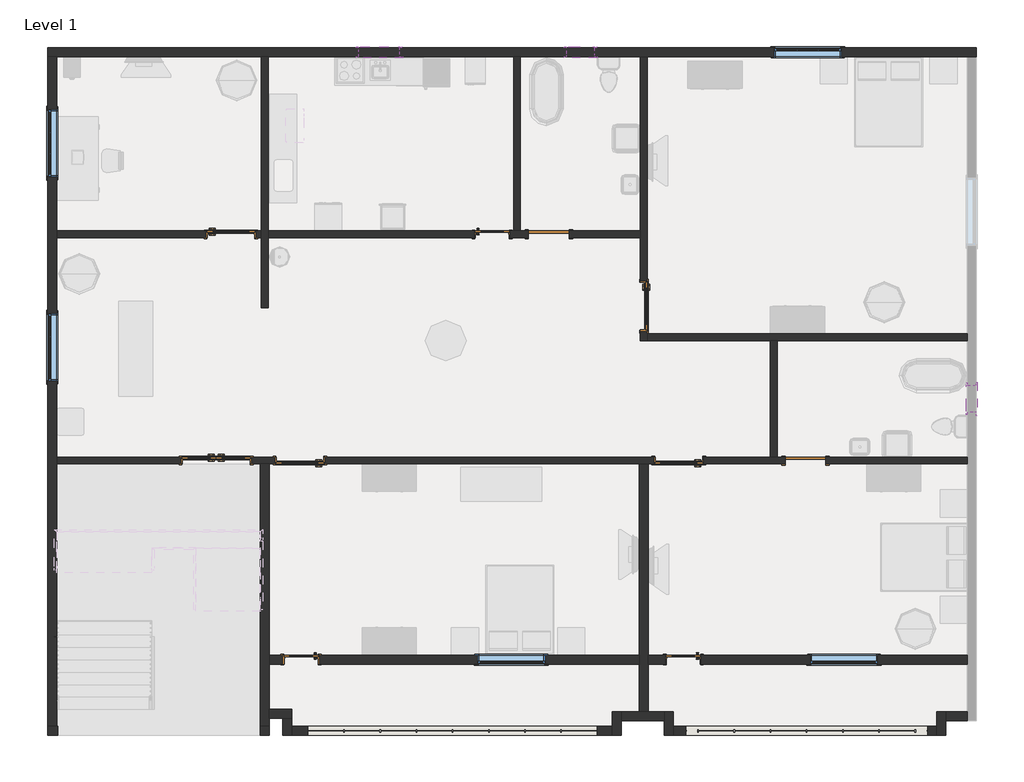
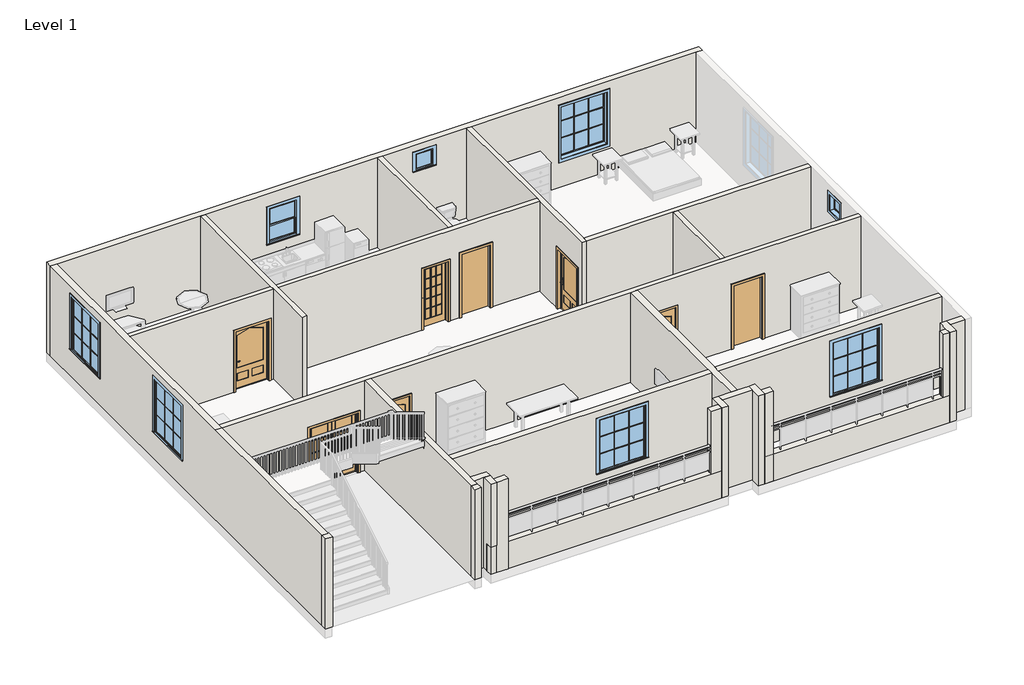
# One storey, part 1 of 4: 27 walls, 10 doors, 8 windows.
"""IFC4 building model written with IfcOpenShell, lengths in millimetres."""

from ifc_helpers import new_model, si_unit, frame, origin, origin_with_axes, place, context, project, spatial, polyline, outline, extrude, faceted_brep, transform, mapped, element, save
from components import door_25c67de5, door_94998e6c, door_d788789e, door_fa41f557, door_686f89d2, window_cc15f82e, window_1554aedb, window_e41d21a6

model = new_model("IFC4")

# Units and contexts
model_context = context("Model", 3, world=origin())
ifc_project = project(units=[si_unit("LENGTHUNIT", "METRE", prefix="MILLI")], contexts=[model_context])

# Site, building, storey
site = spatial("IfcSite", under=ifc_project)
building = spatial("IfcBuilding", under=site)
storey = spatial("IfcBuildingStorey", under=building, Name="Level 1", Elevation=0.0)

# Doors
placement = place(None, origin())
door_shape = door_25c67de5(model_context)
element("IfcDoor", 1, ObjectType="42\" x 80\"", at=placement, inside=storey, context=model_context, shape_type="MappedRepresentation", body=[
    mapped(door_shape, transform((-14516.2480019, 5391.0508877, 0.0), x_axis=(1.0, 0.0, 0.0), y_axis=(0.0, 1.0, 0.0), z_axis=(0.0, 0.0, 1.0))),
])
element("IfcDoor", 2, ObjectType="42\" x 80\"", at=placement, inside=storey, context=model_context, shape_type="MappedRepresentation", body=[
    mapped(door_shape, transform((-6007.2480019, 5391.0508877, 0.0), x_axis=(1.0, 0.0, 0.0), y_axis=(0.0, 1.0, 0.0), z_axis=(0.0, 0.0, 1.0))),
])
element("IfcDoor", 3, ObjectType="42\" x 80\"", at=placement, inside=storey, context=model_context, shape_type="MappedRepresentation", body=[
    mapped(door_shape, transform((-16065.6480019, 10477.4008877, 0.0), x_axis=(-1.0, 0.0, 0.0), y_axis=(0.0, -1.0, 0.0), z_axis=(0.0, 0.0, 1.0))),
])
element("IfcDoor", 4, ObjectType="42\" x 80\"", at=placement, inside=storey, context=model_context, shape_type="MappedRepresentation", body=[
    mapped(door_shape, transform((-6791.4730019, 8861.3258877, 0.0), x_axis=(0.0, 1.0, 0.0), y_axis=(-1.0, 0.0, 0.0), z_axis=(0.0, 0.0, 1.0))),
])
door_2_shape = door_94998e6c(model_context)
element("IfcDoor", 5, ObjectType="Door-Exterior-Double-Full Glass-Wood_Clad : 60\" x 80\"", at=placement, inside=storey, context=model_context, shape_type="MappedRepresentation", body=[
    mapped(door_2_shape, transform((-16395.8480019, 5397.4008877, 0.0), x_axis=(1.0, 0.0, 0.0), y_axis=(0.0, 1.0, 0.0), z_axis=(0.0, 0.0, 1.0))),
])
door_3_shape = door_d788789e(model_context)
element("IfcDoor", 6, ObjectType="Door-Interior-Single-Full Glass-Wood : 30\" x 80\"", at=placement, inside=storey, context=model_context, shape_type="MappedRepresentation", body=[
    mapped(door_3_shape, transform((-14490.8480019, 927.0008877, 0.0), x_axis=(-1.0, 0.0, 0.0), y_axis=(0.0, -1.0, 0.0), z_axis=(0.0, 0.0, 1.0))),
])
element("IfcDoor", 7, ObjectType="Door-Interior-Single-Full Glass-Wood : 30\" x 80\"", at=placement, inside=storey, context=model_context, shape_type="MappedRepresentation", body=[
    mapped(door_3_shape, transform((-5905.6480019, 927.0008877, 0.0), x_axis=(-1.0, 0.0, 0.0), y_axis=(0.0, -1.0, 0.0), z_axis=(0.0, 0.0, 1.0))),
])
door_4_shape = door_fa41f557(model_context)
element("IfcDoor", 8, ObjectType="Door-Interior-Single-Full Glass-Wood : 30\" x 80\"", at=placement, inside=storey, context=model_context, shape_type="MappedRepresentation", body=[
    mapped(door_4_shape, transform((-10198.2480019, 10477.4008877, 0.0), x_axis=(1.0, 0.0, 0.0), y_axis=(0.0, 1.0, 0.0), z_axis=(0.0, 0.0, 1.0))),
])
door_5_shape = door_686f89d2(model_context)
element("IfcDoor", 9, ObjectType="Single-Flush : 36\" x 84\"", at=placement, inside=storey, context=model_context, shape_type="MappedRepresentation", body=[
    mapped(door_5_shape, transform((-8928.2480019, 10474.2258877, 0.0), x_axis=(-1.0, 0.0, 0.0), y_axis=(0.0, -1.0, 0.0), z_axis=(0.0, 0.0, 1.0))),
])
element("IfcDoor", 10, ObjectType="Single-Flush : 36\" x 84\"", at=placement, inside=storey, context=model_context, shape_type="MappedRepresentation", body=[
    mapped(door_5_shape, transform((-3162.4480019, 5394.2258877, 0.0), x_axis=(-1.0, 0.0, 0.0), y_axis=(0.0, -1.0, 0.0), z_axis=(0.0, 0.0, 1.0))),
])

# Walls
element("IfcWall", 11, ObjectType="Generic - 8\"", at=placement, inside=storey, context=model_context, shape_type="Brep", body=[
    faceted_brep([(-20180.4480019, 14462.0258877, 0.0), (-19977.2480019, 14462.0258877, 0.0), (-15379.8480019, 14462.0258877, 0.0), (-15227.4480019, 14462.0258877, 0.0), (-9715.6480019, 14462.0258877, 0.0), (-9563.2480019, 14462.0258877, 0.0), (-6870.8480019, 14462.0258877, 0.0), (-6718.4480019, 14462.0258877, 0.0), (469.7519981, 14462.0258877, 0.0), (672.9519981, 14462.0258877, 0.0), (672.9519981, 14462.0258877, 3048.0), (469.7519981, 14462.0258877, 3048.0), (-6718.4480019, 14462.0258877, 3048.0), (-6870.8480019, 14462.0258877, 3048.0), (-9563.2480019, 14462.0258877, 3048.0), (-9715.6480019, 14462.0258877, 3048.0), (-15227.4480019, 14462.0258877, 3048.0), (-15379.8480019, 14462.0258877, 3048.0), (-19977.2480019, 14462.0258877, 3048.0), (-20180.4480019, 14462.0258877, 3048.0), (-2349.6480019, 14462.0258877, 2743.2), (-2349.6480019, 14462.0258877, 914.4), (-3873.6480019, 14462.0258877, 914.4), (-3873.6480019, 14462.0258877, 2743.2), (-8521.8480019, 14462.0258877, 2768.6), (-7912.2480019, 14462.0258877, 2768.6), (-7912.2480019, 14462.0258877, 2159.0), (-8521.8480019, 14462.0258877, 2159.0), (-13195.4480019, 14462.0258877, 2554.7223406), (-12281.0480019, 14462.0258877, 2554.7223406), (-12281.0480019, 14462.0258877, 1335.5223406), (-13195.4480019, 14462.0258877, 1335.5223406), (-20180.4480019, 14665.2258877, 0.0), (-20180.4480019, 14665.2258877, 3048.0), (672.9519981, 14665.2258877, 3048.0), (672.9519981, 14665.2258877, 0.0), (-2349.6480019, 14665.2258877, 2743.2), (-3873.6480019, 14665.2258877, 2743.2), (-3873.6480019, 14665.2258877, 914.4), (-2349.6480019, 14665.2258877, 914.4), (-8521.8480019, 14665.2258877, 2768.6), (-8521.8480019, 14665.2258877, 2159.0), (-7912.2480019, 14665.2258877, 2159.0), (-7912.2480019, 14665.2258877, 2768.6), (-13195.4480019, 14665.2258877, 2554.7223406), (-13195.4480019, 14665.2258877, 1335.5223406), (-12281.0480019, 14665.2258877, 1335.5223406), (-12281.0480019, 14665.2258877, 2554.7223406)], [[[0, 1, 2, 3, 4, 5, 6, 7, 8, 9, 10, 11, 12, 13, 14, 15, 16, 17, 18, 19], [20, 21, 22, 23], [24, 25, 26, 27], [28, 29, 30, 31]], [[32, 33, 34, 35], [36, 37, 38, 39], [40, 41, 42, 43], [44, 45, 46, 47]], [[9, 8, 7, 6, 5, 4, 3, 2, 1, 0, 32, 35]], [[0, 19, 33, 32]], [[10, 9, 35, 34]], [[21, 20, 36, 39]], [[22, 21, 39, 38]], [[23, 22, 38, 37]], [[20, 23, 37, 36]], [[41, 40, 24, 27]], [[42, 41, 27, 26]], [[43, 42, 26, 25]], [[40, 43, 25, 24]], [[45, 44, 28, 31]], [[46, 45, 31, 30]], [[47, 46, 30, 29]], [[44, 47, 29, 28]], [[19, 18, 17, 16, 15, 14, 13, 12, 11, 10, 34, 33]]]),
])
element("IfcWall", 12, ObjectType="Generic - 8\"", at=placement, inside=storey, context=model_context, shape_type="Brep", body=[
    faceted_brep([(-19977.2480019, -574.7741123, 0.0), (-19977.2480019, 5318.0258877, 0.0), (-19977.2480019, 5470.4258877, 0.0), (-19977.2480019, 10398.0258877, 0.0), (-19977.2480019, 10550.4258877, 0.0), (-19977.2480019, 14462.0258877, 0.0), (-19977.2480019, 14462.0258877, 3048.0), (-19977.2480019, 10550.4258877, 3048.0), (-19977.2480019, 10398.0258877, 3048.0), (-19977.2480019, 5470.4258877, 3048.0), (-19977.2480019, 5318.0258877, 3048.0), (-19977.2480019, -574.7741123, 3048.0), (-19977.2480019, 13280.9258877, 2743.2), (-19977.2480019, 13280.9258877, 914.4), (-19977.2480019, 11756.9258877, 914.4), (-19977.2480019, 11756.9258877, 2743.2), (-19977.2480019, 8696.2258877, 2743.2), (-19977.2480019, 8696.2258877, 914.4), (-19977.2480019, 7172.2258877, 914.4), (-19977.2480019, 7172.2258877, 2743.2), (-20180.4480019, -574.7741123, 0.0), (-20180.4480019, -574.7741123, 3048.0), (-20180.4480019, 5318.0258877, 3048.0), (-20180.4480019, 14462.0258877, 3048.0), (-20180.4480019, 14462.0258877, 0.0), (-20180.4480019, 13280.9258877, 2743.2), (-20180.4480019, 11756.9258877, 2743.2), (-20180.4480019, 11756.9258877, 914.4), (-20180.4480019, 13280.9258877, 914.4), (-20180.4480019, 8696.2258877, 2743.2), (-20180.4480019, 7172.2258877, 2743.2), (-20180.4480019, 7172.2258877, 914.4), (-20180.4480019, 8696.2258877, 914.4)], [[[0, 1, 2, 3, 4, 5, 6, 7, 8, 9, 10, 11], [12, 13, 14, 15], [16, 17, 18, 19]], [[20, 21, 22, 23, 24], [25, 26, 27, 28], [29, 30, 31, 32]], [[5, 4, 3, 2, 1, 0, 20, 24]], [[6, 5, 24, 23]], [[0, 11, 21, 20]], [[13, 12, 25, 28]], [[14, 13, 28, 27]], [[15, 14, 27, 26]], [[12, 15, 26, 25]], [[17, 16, 29, 32]], [[18, 17, 32, 31]], [[19, 18, 31, 30]], [[16, 19, 30, 29]], [[11, 10, 22, 21]], [[10, 9, 8, 7, 6, 23, 22]]]),
])
element("IfcWall", 13, ObjectType="Generic - 8\"", at=placement, inside=storey, context=model_context, shape_type="Brep", body=[
    faceted_brep([(-15202.0480019, -574.7741123, 0.0), (-15202.0480019, -396.9741123, 0.0), (-15202.0480019, -193.7741123, 0.0), (-15202.0480019, 822.2258877, 0.0), (-15202.0480019, 1025.4258877, 0.0), (-15202.0480019, 5318.0258877, 0.0), (-15202.0480019, 5318.0258877, 3048.0), (-15202.0480019, 1025.4258877, 3048.0), (-15202.0480019, 822.2258877, 3048.0), (-15202.0480019, -193.7741123, 3048.0), (-15202.0480019, -396.9741123, 3048.0), (-15202.0480019, -574.7741123, 3048.0), (-15405.2480019, -574.7741123, 0.0), (-15405.2480019, -574.7741123, 3048.0), (-15405.2480019, 5318.0258877, 3048.0), (-15405.2480019, 5318.0258877, 0.0)], [[[0, 1, 2, 3, 4, 5, 6, 7, 8, 9, 10, 11]], [[12, 13, 14, 15]], [[5, 4, 3, 2, 1, 0, 12, 15]], [[0, 11, 13, 12]], [[6, 5, 15, 14]], [[11, 10, 9, 8, 7, 6, 14, 13]]]),
])
element("IfcWall", 14, ObjectType="Generic - 8\"", at=placement, inside=storey, context=model_context, shape_type="SweptSolid", body=[
    extrude(outline(polyline([(3048.0, -15202.0480019), (0.0, -15202.0480019), (0.0, -14897.2480019), (2057.4, -14897.2480019), (2057.4, -14084.4480019), (0.0, -14084.4480019), (0.0, -6896.2480019), (3048.0, -6896.2480019), (3048.0, -15202.0480019)]), holes=[polyline([(914.4, -10528.4480019), (2743.2, -10528.4480019), (2743.2, -9004.4480019), (914.4, -9004.4480019), (914.4, -10528.4480019)])]), frame((0.0, 822.2258877, 0.0), z_axis=(0.0, 1.0, 0.0), x_axis=(0.0, 0.0, 1.0)), (0.0, 0.0, 1.0), 203.2),
    extrude(outline(polyline([(0.0, 469.7519981), (3048.0, 469.7519981), (3048.0, -6693.0480019), (0.0, -6693.0480019), (0.0, -6312.0480019), (2057.4, -6312.0480019), (2057.4, -5499.2480019), (0.0, -5499.2480019), (0.0, 469.7519981)]), holes=[polyline([(914.4, -3060.8480019), (2743.2, -3060.8480019), (2743.2, -1536.8480019), (914.4, -1536.8480019), (914.4, -3060.8480019)])]), frame((0.0, 822.2258877, 0.0), z_axis=(0.0, 1.0, 0.0), x_axis=(0.0, 0.0, 1.0)), (0.0, 0.0, 1.0), 203.2),
])
element("IfcWall", 15, ObjectType="Generic - 8\"", at=placement, inside=storey, context=model_context, shape_type="Brep", body=[
    faceted_brep([(-15202.0480019, -396.9741123, 0.0), (-14897.2480019, -396.9741123, 0.0), (-14694.0480019, -396.9741123, 0.0), (-14694.0480019, -396.9741123, 3048.0), (-14897.2480019, -396.9741123, 3048.0), (-15202.0480019, -396.9741123, 3048.0), (-15202.0480019, -193.7741123, 0.0), (-15202.0480019, -193.7741123, 3048.0), (-14694.0480019, -193.7741123, 3048.0), (-14694.0480019, -193.7741123, 0.0)], [[[0, 1, 2, 3, 4, 5]], [[6, 7, 8, 9]], [[2, 1, 0, 6, 9]], [[0, 5, 7, 6]], [[3, 2, 9, 8]], [[5, 4, 3, 8, 7]]]),
])
element("IfcWall", 16, ObjectType="Generic - 8\"", at=placement, inside=storey, context=model_context, shape_type="Brep", body=[
    faceted_brep([(-14897.2480019, -396.9741123, 0.0), (-14897.2480019, -574.7741123, 0.0), (-14897.2480019, -574.7741123, 914.4), (-14897.2480019, -777.9741123, 914.4), (-14897.2480019, -777.9741123, 3048.0), (-14897.2480019, -396.9741123, 3048.0), (-14694.0480019, -396.9741123, 0.0), (-14694.0480019, -396.9741123, 3048.0), (-14694.0480019, -574.7741123, 3048.0), (-14694.0480019, -777.9741123, 3048.0), (-14694.0480019, -777.9741123, 914.4), (-14694.0480019, -574.7741123, 914.4), (-14694.0480019, -574.7741123, 0.0)], [[[0, 1, 2, 3, 4, 5]], [[6, 7, 8, 9, 10, 11, 12]], [[1, 0, 6, 12]], [[0, 5, 7, 6]], [[10, 3, 2, 11]], [[2, 1, 12, 11]], [[4, 3, 10, 9]], [[5, 4, 9, 8, 7]]]),
])
element("IfcWall", 17, ObjectType="Generic - 8\"", at=placement, inside=storey, context=model_context, shape_type="SweptSolid", body=[
    extrude(outline(polyline([(-15405.2480019, -574.7741123), (-15202.0480019, -574.7741123), (-15202.0480019, -777.9741123), (-15405.2480019, -777.9741123), (-15405.2480019, -574.7741123)])), origin_with_axes(), (0.0, 0.0, 1.0), 3048.0),
])
element("IfcWall", 18, ObjectType="Generic - 8\"", at=placement, inside=storey, context=model_context, shape_type="Brep", body=[
    faceted_brep([(-7302.6480019, -777.9741123, 3048.0), (-7302.6480019, -777.9741123, 0.0), (-7302.6480019, -447.7741123, 0.0), (-7302.6480019, -244.5741123, 0.0), (-7302.6480019, -244.5741123, 3048.0), (-7302.6480019, -447.7741123, 3048.0), (-7505.8480019, -777.9741123, 0.0), (-7505.8480019, -777.9741123, 914.4), (-7505.8480019, -777.9741123, 3048.0), (-7505.8480019, -574.7741123, 3048.0), (-7505.8480019, -244.5741123, 3048.0), (-7505.8480019, -244.5741123, 0.0), (-7505.8480019, -574.7741123, 0.0)], [[[0, 1, 2, 3, 4, 5]], [[6, 7, 8, 9, 10, 11, 12]], [[3, 2, 1, 6, 12, 11]], [[4, 3, 11, 10]], [[0, 8, 7, 6, 1]], [[0, 5, 4, 10, 9, 8]]]),
])
element("IfcWall", 19, ObjectType="Generic - 8\"", at=placement, inside=storey, context=model_context, shape_type="Brep", body=[
    faceted_brep([(-7302.6480019, -447.7741123, 0.0), (-6337.4480019, -447.7741123, 0.0), (-6337.4480019, -447.7741123, 3048.0), (-7302.6480019, -447.7741123, 3048.0), (-7302.6480019, -244.5741123, 0.0), (-7302.6480019, -244.5741123, 3048.0), (-6896.2480019, -244.5741123, 3048.0), (-6693.0480019, -244.5741123, 3048.0), (-6337.4480019, -244.5741123, 3048.0), (-6337.4480019, -244.5741123, 0.0), (-6693.0480019, -244.5741123, 0.0), (-6896.2480019, -244.5741123, 0.0)], [[[0, 1, 2, 3]], [[4, 5, 6, 7, 8, 9, 10, 11]], [[1, 0, 4, 11, 10, 9]], [[0, 3, 5, 4]], [[2, 1, 9, 8]], [[3, 2, 8, 7, 6, 5]]]),
])
element("IfcWall", 20, ObjectType="Generic - 8\"", at=placement, inside=storey, context=model_context, shape_type="Brep", body=[
    faceted_brep([(-6337.4480019, -244.5741123, 0.0), (-6337.4480019, -447.7741123, 0.0), (-6337.4480019, -777.9741123, 0.0), (-6337.4480019, -777.9741123, 3048.0), (-6337.4480019, -447.7741123, 3048.0), (-6337.4480019, -244.5741123, 3048.0), (-6134.2480019, -244.5741123, 0.0), (-6134.2480019, -244.5741123, 3048.0), (-6134.2480019, -574.7741123, 3048.0), (-6134.2480019, -777.9741123, 3048.0), (-6134.2480019, -777.9741123, 914.4), (-6134.2480019, -777.9741123, 0.0), (-6134.2480019, -574.7741123, 0.0)], [[[0, 1, 2, 3, 4, 5]], [[6, 7, 8, 9, 10, 11, 12]], [[2, 1, 0, 6, 12, 11]], [[0, 5, 7, 6]], [[2, 11, 10, 9, 3]], [[5, 4, 3, 9, 8, 7]]]),
])
element("IfcWall", 21, ObjectType="Generic - 8\"", at=placement, inside=storey, context=model_context, shape_type="Brep", body=[
    faceted_brep([(-7505.8480019, -574.7741123, 0.0), (-14694.0480019, -574.7741123, 0.0), (-14897.2480019, -574.7741123, 0.0), (-14897.2480019, -574.7741123, 914.4), (-14694.0480019, -574.7741123, 914.4), (-7505.8480019, -574.7741123, 914.4), (-7505.8480019, -777.9741123, 0.0), (-7505.8480019, -777.9741123, 914.4), (-14694.0480019, -777.9741123, 914.4), (-14897.2480019, -777.9741123, 914.4), (-14897.2480019, -777.9741123, 0.0)], [[[0, 1, 2, 3, 4, 5]], [[6, 7, 8, 9, 10]], [[2, 1, 0, 6, 10]], [[5, 4, 3, 9, 8, 7]], [[3, 2, 10, 9]], [[0, 5, 7, 6]]]),
])
element("IfcWall", 22, ObjectType="Generic - 8\"", at=placement, inside=storey, context=model_context, shape_type="Brep", body=[
    faceted_brep([(-12.8480019, -777.9741123, 3048.0), (-12.8480019, -777.9741123, 0.0), (-12.8480019, -447.7741123, 0.0), (-12.8480019, -244.5741123, 0.0), (-12.8480019, -244.5741123, 3048.0), (-12.8480019, -447.7741123, 3048.0), (-216.0480019, -777.9741123, 0.0), (-216.0480019, -777.9741123, 914.4), (-216.0480019, -777.9741123, 3048.0), (-216.0480019, -574.7741123, 3048.0), (-216.0480019, -244.5741123, 3048.0), (-216.0480019, -244.5741123, 0.0), (-216.0480019, -574.7741123, 0.0)], [[[0, 1, 2, 3, 4, 5]], [[6, 7, 8, 9, 10, 11, 12]], [[3, 2, 1, 6, 12, 11]], [[4, 3, 11, 10]], [[0, 8, 7, 6, 1]], [[0, 5, 4, 10, 9, 8]]]),
])
element("IfcWall", 23, ObjectType="Generic - 8\"", at=placement, inside=storey, context=model_context, shape_type="SweptSolid", body=[
    extrude(outline(polyline([(469.7519981, -447.7741123), (-12.8480019, -447.7741123), (-12.8480019, -244.5741123), (469.7519981, -244.5741123), (469.7519981, -447.7741123)])), origin_with_axes(), (0.0, 0.0, 1.0), 3048.0),
])
element("IfcWall", 24, ObjectType="Generic - 8\"", at=placement, inside=storey, context=model_context, shape_type="SweptSolid", body=[
    extrude(outline(polyline([(-6134.2480019, -574.7741123), (-216.0480019, -574.7741123), (-216.0480019, -777.9741123), (-6134.2480019, -777.9741123), (-6134.2480019, -574.7741123)])), origin_with_axes(), (0.0, 0.0, 1.0), 914.4),
])
element("IfcWall", 25, ObjectType="Generic - 8\"", at=placement, inside=storey, context=model_context, shape_type="Brep", body=[
    faceted_brep([(-6896.2480019, 5318.0258877, 0.0), (-6896.2480019, 1025.4258877, 0.0), (-6896.2480019, 822.2258877, 0.0), (-6896.2480019, -244.5741123, 0.0), (-6896.2480019, -244.5741123, 3048.0), (-6896.2480019, 822.2258877, 3048.0), (-6896.2480019, 1025.4258877, 3048.0), (-6896.2480019, 5318.0258877, 3048.0), (-6693.0480019, 5318.0258877, 0.0), (-6693.0480019, 5318.0258877, 3048.0), (-6693.0480019, 1025.4258877, 3048.0), (-6693.0480019, 822.2258877, 3048.0), (-6693.0480019, -244.5741123, 3048.0), (-6693.0480019, -244.5741123, 0.0), (-6693.0480019, 822.2258877, 0.0), (-6693.0480019, 1025.4258877, 0.0)], [[[0, 1, 2, 3, 4, 5, 6, 7]], [[8, 9, 10, 11, 12, 13, 14, 15]], [[3, 2, 1, 0, 8, 15, 14, 13]], [[4, 3, 13, 12]], [[0, 7, 9, 8]], [[7, 6, 5, 4, 12, 11, 10, 9]]]),
])
element("IfcWall", 26, ObjectType="Generic - 8\"", at=placement, inside=storey, context=model_context, shape_type="Brep", body=[
    faceted_brep([(-19951.8480019, -574.7741123, 0.0), (-19977.2480019, -574.7741123, 0.0), (-20180.4480019, -574.7741123, 0.0), (-20180.4480019, -574.7741123, 3048.0), (-19977.2480019, -574.7741123, 3048.0), (-19951.8480019, -574.7741123, 3048.0), (-19951.8480019, -777.9741123, 0.0), (-19951.8480019, -777.9741123, 3048.0), (-20180.4480019, -777.9741123, 3048.0), (-20180.4480019, -777.9741123, 0.0)], [[[0, 1, 2, 3, 4, 5]], [[6, 7, 8, 9]], [[2, 1, 0, 6, 9]], [[5, 4, 3, 8, 7]], [[0, 5, 7, 6]], [[3, 2, 9, 8]]]),
])
element("IfcWall", 27, ObjectType="Generic - 8\"", at=placement, inside=storey, context=model_context, shape_type="Brep", body=[
    faceted_brep([(-14694.0480019, -777.9741123, 3048.0), (-14694.0480019, -777.9741123, 914.4), (-14694.0480019, -777.9741123, 0.0), (-14338.4480019, -777.9741123, 0.0), (-14338.4480019, -777.9741123, 3048.0), (-14694.0480019, -574.7741123, 0.0), (-14694.0480019, -574.7741123, 3048.0), (-14338.4480019, -574.7741123, 3048.0), (-14338.4480019, -574.7741123, 0.0)], [[[0, 1, 2, 3, 4]], [[5, 6, 7, 8]], [[3, 2, 5, 8]], [[4, 3, 8, 7]], [[0, 6, 5, 2, 1]], [[0, 4, 7, 6]]]),
])
element("IfcWall", 28, ObjectType="Generic - 8\"", at=placement, inside=storey, context=model_context, shape_type="SweptSolid", body=[
    extrude(outline(polyline([(-7836.0480019, -574.7741123), (-7505.8480019, -574.7741123), (-7505.8480019, -777.9741123), (-7836.0480019, -777.9741123), (-7836.0480019, -574.7741123)])), origin_with_axes(), (0.0, 0.0, 1.0), 3048.0),
])
element("IfcWall", 29, ObjectType="Generic - 8\"", at=placement, inside=storey, context=model_context, shape_type="SweptSolid", body=[
    extrude(outline(polyline([(-5854.8480019, -777.9741123), (-6134.2480019, -777.9741123), (-6134.2480019, -574.7741123), (-5854.8480019, -574.7741123), (-5854.8480019, -777.9741123)])), origin_with_axes(), (0.0, 0.0, 1.0), 3048.0),
])
element("IfcWall", 30, ObjectType="Generic - 8\"", at=placement, inside=storey, context=model_context, shape_type="SweptSolid", body=[
    extrude(outline(polyline([(-419.2480019, -574.7741123), (-216.0480019, -574.7741123), (-216.0480019, -777.9741123), (-419.2480019, -777.9741123), (-419.2480019, -574.7741123)])), origin_with_axes(), (0.0, 0.0, 1.0), 3048.0),
])
element("IfcWall", 31, ObjectType="INNER WALL", at=placement, inside=storey, context=model_context, shape_type="Brep", body=[
    faceted_brep([(-19977.2480019, 5318.0258877, 3048.0), (-19977.2480019, 5318.0258877, 0.0), (-17183.2480019, 5318.0258877, 0.0), (-17183.2480019, 5318.0258877, 2057.4), (-15608.4480019, 5318.0258877, 2057.4), (-15608.4480019, 5318.0258877, 0.0), (-15405.2480019, 5318.0258877, 0.0), (-15202.0480019, 5318.0258877, 0.0), (-15075.0480019, 5318.0258877, 0.0), (-15075.0480019, 5318.0258877, 2057.4), (-13957.4480019, 5318.0258877, 2057.4), (-13957.4480019, 5318.0258877, 0.0), (-6896.2480019, 5318.0258877, 0.0), (-6693.0480019, 5318.0258877, 0.0), (-6566.0480019, 5318.0258877, 0.0), (-6566.0480019, 5318.0258877, 2057.4), (-5448.4480019, 5318.0258877, 2057.4), (-5448.4480019, 5318.0258877, 0.0), (-3619.6480019, 5318.0258877, 0.0), (-3619.6480019, 5318.0258877, 2133.6), (-2705.2480019, 5318.0258877, 2133.6), (-2705.2480019, 5318.0258877, 0.0), (469.7519981, 5318.0258877, 0.0), (469.7519981, 5318.0258877, 3048.0), (-6693.0480019, 5318.0258877, 3048.0), (-6896.2480019, 5318.0258877, 3048.0), (-15202.0480019, 5318.0258877, 3048.0), (-15405.2480019, 5318.0258877, 3048.0), (-19977.2480019, 5470.4258877, 3048.0), (-3949.8480019, 5470.4258877, 3048.0), (-3797.4480019, 5470.4258877, 3048.0), (469.7519981, 5470.4258877, 3048.0), (469.7519981, 5470.4258877, 0.0), (-2705.2480019, 5470.4258877, 0.0), (-2705.2480019, 5470.4258877, 2133.6), (-3619.6480019, 5470.4258877, 2133.6), (-3619.6480019, 5470.4258877, 0.0), (-3797.4480019, 5470.4258877, 0.0), (-3949.8480019, 5470.4258877, 0.0), (-5448.4480019, 5470.4258877, 0.0), (-5448.4480019, 5470.4258877, 2057.4), (-6566.0480019, 5470.4258877, 2057.4), (-6566.0480019, 5470.4258877, 0.0), (-13957.4480019, 5470.4258877, 0.0), (-13957.4480019, 5470.4258877, 2057.4), (-15075.0480019, 5470.4258877, 2057.4), (-15075.0480019, 5470.4258877, 0.0), (-15608.4480019, 5470.4258877, 0.0), (-15608.4480019, 5470.4258877, 2057.4), (-17183.2480019, 5470.4258877, 2057.4), (-17183.2480019, 5470.4258877, 0.0), (-19977.2480019, 5470.4258877, 0.0)], [[[0, 1, 2, 3, 4, 5, 6, 7, 8, 9, 10, 11, 12, 13, 14, 15, 16, 17, 18, 19, 20, 21, 22, 23, 24, 25, 26, 27]], [[28, 29, 30, 31, 32, 33, 34, 35, 36, 37, 38, 39, 40, 41, 42, 43, 44, 45, 46, 47, 48, 49, 50, 51]], [[1, 51, 50, 2]], [[32, 22, 21, 33]], [[36, 18, 17, 39, 38, 37]], [[5, 47, 46, 8, 7, 6]], [[11, 43, 42, 14, 13, 12]], [[1, 0, 28, 51]], [[23, 22, 32, 31]], [[19, 18, 36, 35]], [[20, 19, 35, 34]], [[21, 20, 34, 33]], [[4, 48, 47, 5]], [[48, 4, 3, 49]], [[49, 3, 2, 50]], [[10, 44, 43, 11]], [[44, 10, 9, 45]], [[45, 9, 8, 46]], [[16, 40, 39, 17]], [[40, 16, 15, 41]], [[41, 15, 14, 42]], [[31, 30, 29, 28, 0, 27, 26, 25, 24, 23]]]),
])
element("IfcWall", 32, ObjectType="INNER WALL", at=placement, inside=storey, context=model_context, shape_type="Brep", body=[
    faceted_brep([(-19977.2480019, 10398.0258877, 3048.0), (-19977.2480019, 10398.0258877, 0.0), (-16624.4480019, 10398.0258877, 0.0), (-16624.4480019, 10398.0258877, 2057.4), (-15506.8480019, 10398.0258877, 2057.4), (-15506.8480019, 10398.0258877, 0.0), (-15379.8480019, 10398.0258877, 0.0), (-15379.8480019, 10398.0258877, 3048.0), (-19977.2480019, 10550.4258877, 0.0), (-19977.2480019, 10550.4258877, 3048.0), (-15379.8480019, 10550.4258877, 3048.0), (-15379.8480019, 10550.4258877, 0.0), (-15506.8480019, 10550.4258877, 0.0), (-15506.8480019, 10550.4258877, 2057.4), (-16624.4480019, 10550.4258877, 2057.4), (-16624.4480019, 10550.4258877, 0.0)], [[[0, 1, 2, 3, 4, 5, 6, 7]], [[8, 9, 10, 11, 12, 13, 14, 15]], [[1, 8, 15, 2]], [[5, 12, 11, 6]], [[1, 0, 9, 8]], [[7, 6, 11, 10]], [[14, 3, 2, 15]], [[3, 14, 13, 4]], [[4, 13, 12, 5]], [[9, 0, 7, 10]]]),
    faceted_brep([(-6870.8480019, 10398.0258877, 0.0), (-6870.8480019, 10398.0258877, 3048.0), (-15227.4480019, 10398.0258877, 3048.0), (-15227.4480019, 10398.0258877, 0.0), (-10604.6480019, 10398.0258877, 0.0), (-10604.6480019, 10398.0258877, 2057.4), (-9791.8480019, 10398.0258877, 2057.4), (-9791.8480019, 10398.0258877, 0.0), (-9385.4480019, 10398.0258877, 0.0), (-9385.4480019, 10398.0258877, 2133.6), (-8471.0480019, 10398.0258877, 2133.6), (-8471.0480019, 10398.0258877, 0.0), (-6870.8480019, 10550.4258877, 3048.0), (-6870.8480019, 10550.4258877, 0.0), (-8471.0480019, 10550.4258877, 0.0), (-8471.0480019, 10550.4258877, 2133.6), (-9385.4480019, 10550.4258877, 2133.6), (-9385.4480019, 10550.4258877, 0.0), (-9563.2480019, 10550.4258877, 0.0), (-9715.6480019, 10550.4258877, 0.0), (-9791.8480019, 10550.4258877, 0.0), (-9791.8480019, 10550.4258877, 2057.4), (-10604.6480019, 10550.4258877, 2057.4), (-10604.6480019, 10550.4258877, 0.0), (-15227.4480019, 10550.4258877, 0.0), (-15227.4480019, 10550.4258877, 3048.0), (-9715.6480019, 10550.4258877, 3048.0), (-9563.2480019, 10550.4258877, 3048.0)], [[[0, 1, 2, 3, 4, 5, 6, 7, 8, 9, 10, 11]], [[12, 13, 14, 15, 16, 17, 18, 19, 20, 21, 22, 23, 24, 25, 26, 27]], [[13, 0, 11, 14]], [[17, 8, 7, 20, 19, 18]], [[23, 4, 3, 24]], [[1, 0, 13, 12]], [[3, 2, 25, 24]], [[9, 8, 17, 16]], [[10, 9, 16, 15]], [[11, 10, 15, 14]], [[6, 21, 20, 7]], [[21, 6, 5, 22]], [[22, 5, 4, 23]], [[1, 12, 27, 26, 25, 2]]]),
])
element("IfcWall", 33, ObjectType="INNER WALL", at=placement, inside=storey, context=model_context, shape_type="Brep", body=[
    faceted_brep([(469.7519981, 8239.0258877, 0.0), (-6718.4480019, 8239.0258877, 0.0), (-6718.4480019, 8239.0258877, 3048.0), (469.7519981, 8239.0258877, 3048.0), (469.7519981, 8086.6258877, 0.0), (469.7519981, 8086.6258877, 3048.0), (-3797.4480019, 8086.6258877, 3048.0), (-3949.8480019, 8086.6258877, 3048.0), (-6718.4480019, 8086.6258877, 3048.0), (-6718.4480019, 8086.6258877, 0.0), (-3949.8480019, 8086.6258877, 0.0), (-3797.4480019, 8086.6258877, 0.0)], [[[0, 1, 2, 3]], [[4, 5, 6, 7, 8, 9, 10, 11]], [[1, 0, 4, 11, 10, 9]], [[0, 3, 5, 4]], [[2, 1, 9, 8]], [[3, 2, 8, 7, 6, 5]]]),
])
element("IfcWall", 34, ObjectType="INNER WALL", at=placement, inside=storey, context=model_context, shape_type="Brep", body=[
    faceted_brep([(-6870.8480019, 14462.0258877, 3048.0), (-6870.8480019, 14462.0258877, 0.0), (-6870.8480019, 10550.4258877, 0.0), (-6870.8480019, 10398.0258877, 0.0), (-6870.8480019, 9420.1258877, 0.0), (-6870.8480019, 9420.1258877, 2057.4), (-6870.8480019, 8302.5258877, 2057.4), (-6870.8480019, 8302.5258877, 0.0), (-6870.8480019, 8086.6258877, 0.0), (-6870.8480019, 8086.6258877, 3048.0), (-6870.8480019, 10398.0258877, 3048.0), (-6870.8480019, 10550.4258877, 3048.0), (-6718.4480019, 14462.0258877, 0.0), (-6718.4480019, 14462.0258877, 3048.0), (-6718.4480019, 8239.0258877, 3048.0), (-6718.4480019, 8086.6258877, 3048.0), (-6718.4480019, 8086.6258877, 0.0), (-6718.4480019, 8239.0258877, 0.0), (-6718.4480019, 8302.5258877, 0.0), (-6718.4480019, 8302.5258877, 2057.4), (-6718.4480019, 9420.1258877, 2057.4), (-6718.4480019, 9420.1258877, 0.0)], [[[0, 1, 2, 3, 4, 5, 6, 7, 8, 9, 10, 11]], [[12, 13, 14, 15, 16, 17, 18, 19, 20, 21]], [[1, 12, 21, 4, 3, 2]], [[16, 8, 7, 18, 17]], [[1, 0, 13, 12]], [[9, 8, 16, 15]], [[20, 5, 4, 21]], [[5, 20, 19, 6]], [[6, 19, 18, 7]], [[0, 11, 10, 9, 15, 14, 13]]]),
])
element("IfcWall", 35, ObjectType="INNER WALL", at=placement, inside=storey, context=model_context, shape_type="SweptSolid", body=[
    extrude(outline(polyline([(-3949.8480019, 5470.4258877), (-3949.8480019, 8086.6258877), (-3797.4480019, 8086.6258877), (-3797.4480019, 5470.4258877), (-3949.8480019, 5470.4258877)])), origin_with_axes(), (0.0, 0.0, 1.0), 3048.0),
])
element("IfcWall", 36, ObjectType="INNER WALL", at=placement, inside=storey, context=model_context, shape_type="SweptSolid", body=[
    extrude(outline(polyline([(-9715.6480019, 10550.4258877), (-9715.6480019, 14462.0258877), (-9563.2480019, 14462.0258877), (-9563.2480019, 10550.4258877), (-9715.6480019, 10550.4258877)])), origin_with_axes(), (0.0, 0.0, 1.0), 3048.0),
])
element("IfcWall", 37, ObjectType="INNER WALL", at=placement, inside=storey, context=model_context, shape_type="Brep", body=[
    faceted_brep([(-15227.4480019, 8823.2258877, 0.0), (-15227.4480019, 10398.0258877, 0.0), (-15227.4480019, 10550.4258877, 0.0), (-15227.4480019, 14462.0258877, 0.0), (-15227.4480019, 14462.0258877, 3048.0), (-15227.4480019, 10550.4258877, 3048.0), (-15227.4480019, 10398.0258877, 3048.0), (-15227.4480019, 8823.2258877, 3048.0), (-15379.8480019, 8823.2258877, 0.0), (-15379.8480019, 8823.2258877, 3048.0), (-15379.8480019, 10398.0258877, 3048.0), (-15379.8480019, 10550.4258877, 3048.0), (-15379.8480019, 14462.0258877, 3048.0), (-15379.8480019, 14462.0258877, 0.0), (-15379.8480019, 10550.4258877, 0.0), (-15379.8480019, 10398.0258877, 0.0)], [[[0, 1, 2, 3, 4, 5, 6, 7]], [[8, 9, 10, 11, 12, 13, 14, 15]], [[3, 2, 1, 0, 8, 15, 14, 13]], [[0, 7, 9, 8]], [[4, 3, 13, 12]], [[7, 6, 5, 4, 12, 11, 10, 9]]]),
])

# Windows
window_shape = window_cc15f82e(model_context)
element("IfcWindow", 38, ObjectType="Casement 3x3 with Trim : 60\" x 72\"", at=placement, inside=storey, context=model_context, shape_type="MappedRepresentation", body=[
    mapped(window_shape, transform((-9766.4480019, 923.8258877, 609.6), x_axis=(-1.0, 0.0, 0.0), y_axis=(0.0, -1.0, 0.0), z_axis=(0.0, 0.0, 1.0))),
])
element("IfcWindow", 39, ObjectType="Casement 3x3 with Trim : 60\" x 72\"", at=placement, inside=storey, context=model_context, shape_type="MappedRepresentation", body=[
    mapped(window_shape, transform((-2298.8480019, 923.8258877, 609.6), x_axis=(-1.0, 0.0, 0.0), y_axis=(0.0, -1.0, 0.0), z_axis=(0.0, 0.0, 1.0))),
])
element("IfcWindow", 40, ObjectType="Casement 3x3 with Trim : 60\" x 72\"", at=placement, inside=storey, context=model_context, shape_type="MappedRepresentation", body=[
    mapped(window_shape, transform((-3111.6480019, 14563.6258877, 609.6), x_axis=(1.0, 0.0, 0.0), y_axis=(0.0, 1.0, 0.0), z_axis=(0.0, 0.0, 1.0))),
])
element("IfcWindow", 41, ObjectType="Casement 3x3 with Trim : 60\" x 72\"", at=placement, inside=storey, context=model_context, shape_type="MappedRepresentation", body=[
    mapped(window_shape, transform((-20078.8480019, 12518.9258877, 609.6), x_axis=(0.0, 1.0, 0.0), y_axis=(-1.0, 0.0, 0.0), z_axis=(0.0, 0.0, 1.0))),
])
element("IfcWindow", 42, ObjectType="Casement 3x3 with Trim : 60\" x 72\"", at=placement, inside=storey, context=model_context, shape_type="MappedRepresentation", body=[
    mapped(window_shape, transform((-20078.8480019, 7934.2258877, 609.6), x_axis=(0.0, 1.0, 0.0), y_axis=(-1.0, 0.0, 0.0), z_axis=(0.0, 0.0, 1.0))),
])
window_2_shape = window_1554aedb(model_context)
element("IfcWindow", 43, ObjectType="Double Hung with Trim : 36\" x 48\"", at=placement, inside=storey, context=model_context, shape_type="MappedRepresentation", body=[
    mapped(window_2_shape, transform((-12738.2480019, 14563.6258877, 1030.7223406), x_axis=(-1.0, 0.0, 0.0), y_axis=(0.0, -1.0, 0.0), z_axis=(0.0, 0.0, 1.0))),
])
window_3_shape = window_e41d21a6(model_context)
element("IfcWindow", 44, ObjectType="Transom with Trim : 24\" x 24\"", at=placement, inside=storey, context=model_context, shape_type="MappedRepresentation", body=[
    mapped(window_3_shape, transform((-8255.1480019, 14563.6258877, 0.0), x_axis=(-1.0, 0.0, 0.0), y_axis=(0.0, -1.0, 0.0), z_axis=(0.0, 0.0, 1.0))),
])
element("IfcWindow", 45, ObjectType="Transom with Trim : 24\" x 24\"", at=placement, inside=storey, context=model_context, shape_type="MappedRepresentation", body=[
    mapped(window_3_shape, transform((571.3519981, 6740.4258877, 0.0), x_axis=(0.0, -1.0, 0.0), y_axis=(1.0, 0.0, 0.0), z_axis=(0.0, 0.0, 1.0))),
])

save(model, "model.ifc")

# Revit data of these elements
# Type "42\" x 80\""
#   Type Mark = "9"
#   Assembly Code = "B2030100"
#   Analytic Construction = "French door, wood frame with single glass"
#   Threshold Offset [instance default] = 0' - 0 1/2"
#   Thickness = 0' - 1 3/8"
#   Thermal Resistance (R) = 1.0696 (h·ft²·°F)/BTU
#   Swing Angle [instance default] = 90.00°
#   Stiles = 0' - 4 3/4"
#   Rough Width = 3' - 8"
#   Rough Height = 6' - 9"
#   Radius = 2' - 4 29/32"
#   Lock Rail = 0' - 7 1/8"
#   Height = 6' - 8"
#   Width = 3' - 6"
#   Heat Transfer Coefficient (U) = 0.9350 BTU/(h·ft²·°F)
#   Door Offset [instance default] = 0' - 0"
#   Bottom Rail = 0' - 9 1/2"
#   Threshold [instance default] = yes
#   Function = 1
#   Exterior Trim [instance default] = yes
#   Trim Material = Cherry
#   Threshold Material = Cherry
#   Panel Material = Cherry
#   Glazing = Glass
#   Frame Material = Cherry
#   Door Handle Material = Aluminum
#   Visual Light Transmittance = 0
#   Solar Heat Gain Coefficient = 0
#   Wall Closure = (empty or 0)
#   Construction Type = (empty or 0)
# Type "Door-Exterior-Double-Full Glass-Wood_Clad : 60\" x 80\""
#   Type Mark = "8"
#   Assembly Code = "B2030100"
#   Analytic Construction = "French door, wood frame with double glass"
#   Top Rail = 0' - 4 11/16"
#   Threshold Offset [instance default] = 0' - 0 1/2"
#   Thickness = 0' - 1 3/8"
#   Thermal Resistance (R) = 1.9158 (h·ft²·°F)/BTU
#   Swing Angle [instance default] = 90.00°
#   Stiles = 0' - 4 3/4"
#   Rough Width = 5' - 2"
#   Rough Height = 6' - 9"
#   Panel Width = 2' - 6"
#   Door Offset [instance default] = 0' - 0"
#   Height = 6' - 8"
#   Width = 5' - 0"
#   Heat Transfer Coefficient (U) = 0.5220 BTU/(h·ft²·°F)
#   Bottom Rail = 0' - 9 1/8"
#   Exterior Trim [instance default] = yes
#   Threshold [instance default] = yes
#   Show Grill [instance default] = yes
#   Function = 1
#   Trim Material = Cherry
#   Threshold Material = Cherry
#   Panel Material = Cherry
#   Glazing = Glass
#   Frame Material = Cherry
#   Door Handle Material = Aluminum
#   Visual Light Transmittance = 0
#   Solar Heat Gain Coefficient = 0
#   Wall Closure = (empty or 0)
#   Construction Type = (empty or 0)
# Type "Door-Interior-Single-Full Glass-Wood : 30\" x 80\""
#   Type Mark = "10"
#   Assembly Code = "C1020300"
#   Analytic Construction = "Wood frame with single clear glass"
#   Top Rail = 0' - 4 11/16"
#   Thickness = 0' - 1 3/8"
#   Thermal Resistance (R) = 1.0102 (h·ft²·°F)/BTU
#   Swing Angle [instance default] = 90.00°
#   Stiles = 0' - 4 3/4"
#   Rough Width = 2' - 8"
#   Rough Height = 6' - 9"
#   Height = 6' - 8"
#   Width = 2' - 6"
#   Heat Transfer Coefficient (U) = 0.9900 BTU/(h·ft²·°F)
#   Bottom Rail = 0' - 9 1/8"
#   Show Grill [instance default] = yes
#   Trim Material = Cherry
#   Panel Material = Cherry
#   Frame Material = Cherry
#   Door Handle Material = Aluminum
#   Visual Light Transmittance = 0
#   Solar Heat Gain Coefficient = 0
#   Wall Closure = (empty or 0)
#   Function = (empty or 0)
# Type "Single-Flush : 36\" x 84\""
#   Type Mark = "1"
#   Construction Type Id = "MDOOR"
#   Assembly Code = "C1020"
#   Analytic Construction = "Metal"
#   Thickness = 0' - 2"
#   Heat Transfer Coefficient (U) = 0.651978 BTU/(h·ft²·°F)
#   Height = 7' - 0"
#   Trim Projection Ext = 0' - 1"
#   Trim Projection Int = 0' - 1"
#   Trim Width = 0' - 3"
#   Width = 3' - 0"
#   Define Thermal Properties by = 1
#   Door Material = Door - Panel
#   Frame Material = Door - Frame
#   Visual Light Transmittance = 0
#   Solar Heat Gain Coefficient = 0
#   Function = (empty or 0)
#   Wall Closure = (empty or 0)
# Type "Generic - 8\""
#   Assembly Code = "B2010"
#   Layers, outside or top first: 0' - 8" "Brick, Common" (function 1)
# Type "INNER WALL"
#   Assembly Code = "B2010"
#   Layers, outside or top first: 0' - 6" "Brick, Soldier Course" (function 1)
# Type "Casement 3x3 with Trim : 60\" x 72\""
#   Type Mark = "12"
#   Construction Type Id = "GSP4R"
#   Assembly Code = "B2020100"
#   Analytic Construction = "1/8 in Pilkington single glazing"
#   Visual Light Transmittance = 0.9
#   Solar Heat Gain Coefficient = 0.78
#   Heat Transfer Coefficient (U) = 0.6496 BTU/(h·ft²·°F)
#   Height = 6' - 0"
#   Default Sill Height = 1' - 0"
#   Trim Projection - Ext. = 0' - 0 1/2"
#   Trim Projection - Int. = 0' - 0 3/4"
#   Trim Width - Exterior = 0' - 3 1/2"
#   Trim Width - Interior = 0' - 3 1/2"
#   Width = 5' - 0"
#   Window Inset = 0' - 0 3/4"
#   Define Thermal Properties by = 1
#   Glass Pane Material = Glass
#   Sash Material = Sash
#   Trim Exterior Material = Trim
#   Trim Interior Material = Trim
#   Wall Closure = (empty or 0)
# Type "Double Hung with Trim : 36\" x 48\""
#   Type Mark = "21"
#   Construction Type Id = "GSP4R"
#   Assembly Code = "B2020100"
#   Analytic Construction = "1/8 in Pilkington single glazing"
#   Visual Light Transmittance = 0.9
#   Solar Heat Gain Coefficient = 0.78
#   Heat Transfer Coefficient (U) = 0.6496 BTU/(h·ft²·°F)
#   Height = 4' - 0"
#   Default Sill Height = 1' - 0"
#   Trim Projection - Ext. = 0' - 0 1/2"
#   Trim Projection - Int. = 0' - 0 3/4"
#   Trim Width - Exterior = 0' - 3 1/2"
#   Trim Width - Interior = 0' - 3 1/2"
#   Width = 3' - 0"
#   Window Inset = 0' - 0 3/4"
#   Define Thermal Properties by = 1
#   Glass Pane Material = Glass
#   Sash Material = Sash
#   Trim Exterior Material = Trim
#   Trim Interior Material = Trim
#   Wall Closure = (empty or 0)
# Type "Transom with Trim : 24\" x 24\""
#   Type Mark = "22"
#   Construction Type Id = "GSP4R"
#   Assembly Code = "B2020100"
#   Analytic Construction = "1/8 in Pilkington single glazing"
#   Visual Light Transmittance = 0.9
#   Solar Heat Gain Coefficient = 0.78
#   Heat Transfer Coefficient (U) = 0.6496 BTU/(h·ft²·°F)
#   Height = 2' - 0"
#   Default Sill Height = 7' - 1"
#   Trim Projection - Ext. = 0' - 0 1/2"
#   Trim Projection - Int. = 0' - 0 3/4"
#   Trim Width - Exterior = 0' - 3 1/2"
#   Trim Width - Interior = 0' - 3 1/2"
#   Width = 2' - 0"
#   Window Inset = 0' - 0 3/4"
#   Define Thermal Properties by = 1
#   Glass Pane Material = Glass
#   Sash Material = Sash
#   Trim Exterior Material = Trim
#   Trim Interior Material = Trim
#   Wall Closure = (empty or 0)
# Elements 1, 2, 3, 4 (IfcDoor, "42\" x 80\"")
#   Threshold Offset = 0' - 0 1/2"
#   Swing Angle = 90.00°
#   Door Offset = 0' - 0"
#   Threshold = yes
#   Exterior Trim = yes
#   Phase Created = New Construction
#   Materials on its faces: "Cherry", "Aluminum", "Glass"
# Element 5 (IfcDoor, "Door-Exterior-Double-Full Glass-Wood_Clad : 60\" x 80\"")
#   Threshold Offset = 0' - 0 1/2"
#   Swing Angle = 90.00°
#   Door Offset = 0' - 0"
#   Threshold = yes
#   Show Grill = yes
#   Exterior Trim = yes
#   Phase Created = New Construction
#   Materials on its faces: "Cherry", "Aluminum", "Glass"
# Elements 6, 7, 8 (IfcDoor, "Door-Interior-Single-Full Glass-Wood : 30\" x 80\"")
#   Swing Angle = 90.00°
#   Show Grill = yes
#   Phase Created = New Construction
#   Materials on its faces: "Cherry", "Aluminum", "Glass"
# Elements 9, 10 (IfcDoor, "Single-Flush : 36\" x 84\"")
#   Phase Created = New Construction
#   Materials on its faces: "Door - Frame", "Door - Panel"
# Elements 11, 12, 13, 14, 15, 16, 17, 18, 19, 20, 22, 23, 25, 26, 27, 28, 29, 30 (IfcWall, "Generic - 8\"")
#   Top Offset = 0' - 0"
#   Base Offset = 0' - 0"
#   Unconnected Height = 10' - 0"
#   wall height = 10' - 0"
#   Phase Created = New Construction
#   Base Constraint = Level 1
#   Materials on its faces: "Brick, Common"
# Elements 21, 24 (IfcWall, "Generic - 8\"")
#   Top Offset = 0' - 0"
#   Base Offset = 0' - 0"
#   Unconnected Height = 3' - 0"
#   wall height = 3' - 0"
#   Phase Created = New Construction
#   Base Constraint = Level 1
#   Materials on its faces: "Brick, Common"
# Elements 31, 32, 33, 34, 35, 36, 37 (IfcWall, "INNER WALL")
#   Top Offset = 0' - 0"
#   Base Offset = 0' - 0"
#   Unconnected Height = 10' - 0"
#   wall height = 10' - 0"
#   Phase Created = New Construction
#   Base Constraint = Level 1
#   Materials on its faces: "Brick, Soldier Course"
# Element 38 (IfcWindow, "Casement 3x3 with Trim : 60\" x 72\"")
#   Mark = "1"
#   Phase Created = New Construction
#   Materials on its faces: "Sash", "Glass", "Trim"
# Element 39 (IfcWindow, "Casement 3x3 with Trim : 60\" x 72\"")
#   Mark = "2"
#   Phase Created = New Construction
#   Materials on its faces: "Sash", "Glass", "Trim"
# Element 40 (IfcWindow, "Casement 3x3 with Trim : 60\" x 72\"")
#   Mark = "4"
#   Phase Created = New Construction
#   Materials on its faces: "Sash", "Glass", "Trim"
# Element 41 (IfcWindow, "Casement 3x3 with Trim : 60\" x 72\"")
#   Mark = "5"
#   Phase Created = New Construction
#   Materials on its faces: "Sash", "Glass", "Trim"
# Element 42 (IfcWindow, "Casement 3x3 with Trim : 60\" x 72\"")
#   Mark = "6"
#   Phase Created = New Construction
#   Materials on its faces: "Sash", "Glass", "Trim"
# Element 43 (IfcWindow, "Double Hung with Trim : 36\" x 48\"")
#   Mark = "10"
#   Phase Created = New Construction
#   Materials on its faces: "Sash", "Trim", "Glass"
# Element 44 (IfcWindow, "Transom with Trim : 24\" x 24\"")
#   Mark = "8"
#   Phase Created = New Construction
#   Materials on its faces: "Sash", "Trim", "Glass"
# Element 45 (IfcWindow, "Transom with Trim : 24\" x 24\"")
#   Mark = "9"
#   Phase Created = New Construction
#   Materials on its faces: "Sash", "Trim", "Glass"
# Materials
#   "Cherry": class "Wood", colour RGB 226 177 128, transparency 0, Description = "Prunus Serotina", Cost = 0
#   "Glass": class "Glass", colour RGB 0 128 192, transparency 0.75, Description = "Soda Lime Glass", Cost = 0
#   "Aluminum": class "Metal", colour RGB 247 247 247, transparency 0, Description = "Aluminum 6061", Cost = 0
#   "Door - Panel": class "Wood", colour RGB 210 159 95, transparency 0
#   "Door - Frame": colour RGB 118 70 51, transparency 0
#   "Brick, Common": class "Masonry", colour RGB 170 98 104, transparency 0, Description = "Common brick", Cost = 0
#   "Brick, Soldier Course": class "Masonry", colour RGB 170 98 104, transparency 0, Description = "Common brick soldier coursed", Cost = 0
#   "Sash": class "Wood", colour RGB 224 178 126, transparency 0
#   "Trim": class "Wood", colour RGB 224 178 126, transparency 0
# Room at (-17586.338, 12525.226) mm, phase "New Construction", upper level "Level 1", upper offset 10' - 0", lower offset 0' - 0"
#   Number = "1"
# Room at (-12639.732, 12525.226) mm, phase "New Construction", upper level "Level 1", upper offset 10' - 0", lower offset 0' - 0"
#   Number = "2"
#   Name = "KITCHEN"
# Room at (-8235.657, 12525.226) mm, phase "New Construction", upper level "Level 1", upper offset 10' - 0", lower offset 0' - 0"
#   Number = "3"
#   Name = "TOILET"
# Room at (-3129.483, 11695.473) mm, phase "New Construction", upper level "Level 1", upper offset 10' - 0", lower offset 0' - 0"
#   Number = "4"
#   Name = "BED ROOM 1"
# Room at (-1821.026, 7004.175) mm, phase "New Construction", upper level "Level 1", upper offset 10' - 0", lower offset 0' - 0"
#   Number = "5"
#   Name = "TOILET"
# Room at (-17586.338, 7833.929) mm, phase "New Construction", upper level "Level 1", upper offset 10' - 0", lower offset 0' - 0"
#   Number = "6"
#   Name = "DRAWING ROOM"
# Room at (-10810.932, 7833.929) mm, phase "New Construction", upper level "Level 1", upper offset 10' - 0", lower offset 0' - 0"
#   Number = "7"
# Room at (-18001.214, 2344.792) mm, phase "New Construction", upper level "Level 1", upper offset 10' - 0", lower offset 0' - 0"
#   Number = "8"
# Room at (-11363.188, 0) mm, phase "New Construction", upper level "Level 1", upper offset 10' - 0", lower offset 0' - 0"
#   Number = "9"
# Room at (-3129.483, 0) mm, phase "New Construction", upper level "Level 1", upper offset 10' - 0", lower offset 0' - 0"
#   Number = "10"
# Room at (-3129.483, 3606.947) mm, phase "New Construction", upper level "Level 1", upper offset 10' - 0", lower offset 0' - 0"
#   Number = "11"
#   Name = "BED ROOM 3"
# Room at (-11363.188, 3206.459) mm, phase "New Construction", upper level "Level 1", upper offset 10' - 0", lower offset 0' - 0"
#   Number = "12"
#   Name = "BED ROOM 2"
